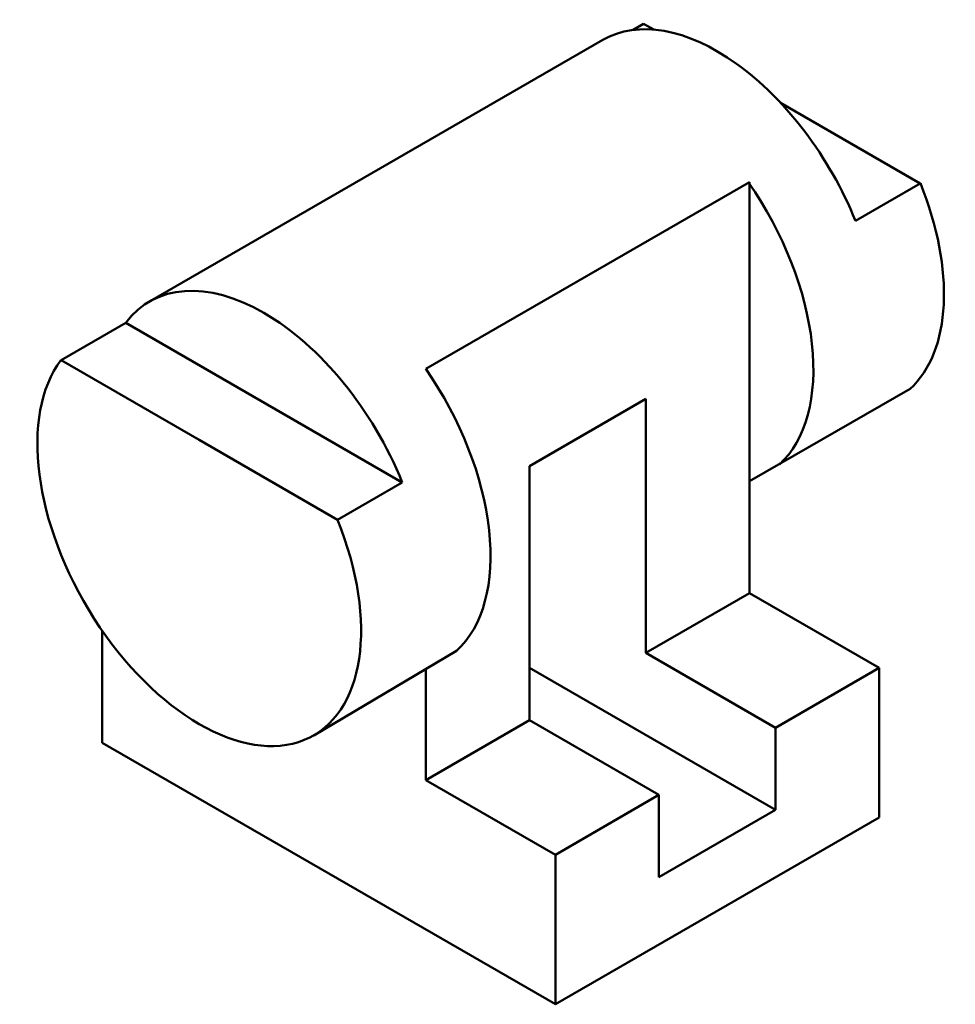
# Model space of a CAD drawing. Units: millimetres. Extents: x 2297 to 2422, y 1542 to 1674.
import ezdxf

# ---------------------------------------------------------------- set-up
doc = ezdxf.new("R2010")
doc.units = ezdxf.units.MM
doc.layers.add('M-OUTL', color=7, linetype='Continuous', lineweight=50)

msp = doc.modelspace()

# ---------------------------------------------------------------- linework, layer by layer
at = {"layer": 'M-OUTL'}
for p, q in [((2379.05, 1672.42), (2380.47, 1673.24)), ((2381.82, 1672.47), (2380.47, 1673.24)), ((2314.38, 1636.08), (2375, 1671.08)), ((2417.46, 1651.89), (2398.79, 1662.67)), ((2394.64, 1652.07), (2351.34, 1627.07)), ((2394.64, 1597.07), (2394.64, 1652.07)), ((2408.8, 1646.89), (2417.46, 1651.89)), ((2417.46, 1651.89), (2417.5, 1651.91)), ((2302.53, 1628.24), (2311.19, 1633.24)), ((2348.18, 1611.89), (2311.19, 1633.24)), ((2321.02, 1617.57), (2302.53, 1628.24)), ((2416.11, 1624.39), (2394.64, 1612.04)), ((2365.19, 1614.07), (2380.78, 1623.07)), ((2380.78, 1623.07), (2380.78, 1589.07)), ((2321.02, 1617.57), (2339.52, 1606.89)), ((2365.19, 1580.07), (2365.19, 1614.07)), ((2339.52, 1606.89), (2348.18, 1611.89)), ((2380.78, 1589.07), (2394.64, 1597.07)), ((2394.64, 1597.07), (2411.96, 1587.07)), ((2308.03, 1577.07), (2308.03, 1592.07)), ((2355.45, 1589.37), (2336.33, 1578.05)), ((2380.78, 1589.07), (2398.1, 1579.07)), ((2351.34, 1572.07), (2351.34, 1586.93)), ((2398.1, 1568.07), (2365.19, 1587.07)), ((2411.96, 1587.07), (2398.1, 1579.07)), ((2411.96, 1567.07), (2411.96, 1587.07)), ((2351.34, 1572.07), (2365.19, 1580.07)), ((2365.19, 1580.07), (2382.51, 1570.07)), ((2398.1, 1579.07), (2398.1, 1568.07)), ((2368.66, 1542.07), (2308.03, 1577.07)), ((2368.66, 1562.07), (2351.34, 1572.07)), ((2382.51, 1570.07), (2368.66, 1562.07)), ((2382.51, 1559.07), (2382.51, 1570.07)), ((2398.1, 1568.07), (2382.51, 1559.07)), ((2368.66, 1542.07), (2411.96, 1567.07)), ((2368.66, 1562.07), (2368.66, 1542.07))]:
    msp.add_line(p, q, dxfattribs=at)
for centre, start_param, end_param in [((2390.31, 1644.57), 7.615434, 9.424778), ((2381.53, 1639.5), 6.40899, 7.995879), ((2399, 1649.59), 6.40899, 7.615434), ((2329.68, 1609.57), 7.615434, 9.663325), ((2321.02, 1604.57), 3.38014, 7.615434), ((2338.34, 1614.57), 6.40899, 7.995879)]:
    msp.add_ellipse(centre, major_axis=(15.31, -26.52), ratio=0.57735, start_param=start_param, end_param=end_param, dxfattribs=at)

doc.saveas('drawing.dxf')
